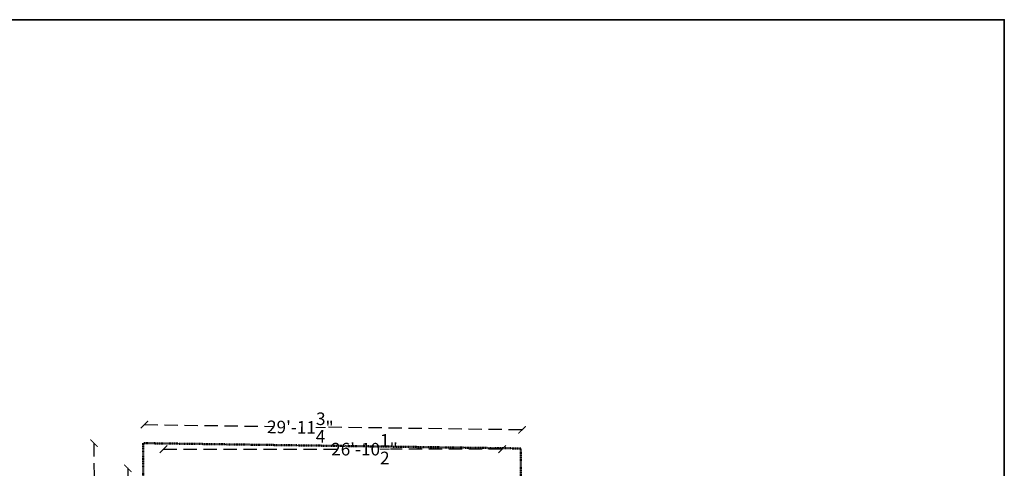
# Model space of a CAD drawing. Units: inches. Extents: x -16911 to -9621, y -48626 to -46270.
# Tile 16 of 20: x -10695 to -9757, y -47771 to -47344. Entities that reach past the tile are written whole.
import ezdxf

# ---------------------------------------------------------------- set-up
doc = ezdxf.new("R2010")
doc.units = ezdxf.units.IN
for name, pattern in [('DASHDOT', [1, 0.5, -0.25, 0, -0.25]), ('DASHED', [19.05, 12.7, -6.35]), ('DOT2', [3.175, 0, -3.175])]:
    doc.linetypes.add(name, pattern=pattern)
for name, color, linetype, lineweight in [('A-ANNO-DIMS', 2, 'Continuous', 13), ('A-WALL', 7, 'Continuous', 35), ('C-PROP', 6, 'DASHDOT', 50)]:
    doc.layers.add(name, color=color, linetype=linetype, lineweight=lineweight)
doc.styles.add('style9', font='swisscl.ttf', dxfattribs={"height": 12})
doc.dimstyles.new('Dim9', dxfattribs={"dimtxt": 10, "dimasz": 0.199219, "dimexe": 1, "dimexo": 0.5, "dimgap": 1, "dimtad": 0, "dimdec": 1, "dimzin": 0, "dimdsep": 46, "dimlunit": 4, "dimtxsty": 'style9', "dimblk": 'ARCHTICK', "dimcen": 0.09, "dimclrd": 256, "dimclrt": 256, "dimadec": 0, "dimazin": 0, "dimtfac": 1, "dimtdec": 1, "dimtix": 1, "dimtofl": 0, "dimtmove": 1, "dimatfit": 3, "dimfxl": 9, "dimtolj": 1, "dimtzin": 0, "dimlwd": -1, "dimarcsym": 0})

# ---------------------------------------------------------------- blocks, each defined once
blk = doc.blocks.new('_ArchTick')
at = {"color": 0, "linetype": 'ByBlock', "const_width": 0.15}
blk.add_lwpolyline([(-0.5, -0.5), (0.5, 0.5)], dxfattribs=at)
blk = doc.blocks.new('*D23')
at = {"layer": 'A-ANNO-DIMS', "color": 0, "linetype": 'DOT2', "lineweight": -2, "transparency": 16777216}
for p, q in [((-10576.06, -47729.98), (-10576.04, -47728.79)), ((-10216.4, -47735.03), (-10216.38, -47733.84))]:
    blk.add_line(p, q, dxfattribs=at)
at = {"layer": 'A-ANNO-DIMS', "color": 0, "linetype": 'DASHED', "lineweight": 25, "transparency": 16777216}
for p, q in [((-10576.06, -47729.79), (-10452.32, -47731.53)), ((-10216.39, -47734.84), (-10402.73, -47732.22))]:
    blk.add_line(p, q, dxfattribs=at)
at = {"layer": 'Defpoints', "color": 0, "transparency": 16777216}
for p in [(-10576.25, -47743.71), (-10216.39, -47734.84), (-10216.59, -47748.75)]:
    blk.add_point(p, dxfattribs=at)
at = {"layer": 'A-ANNO-DIMS', "color": 0, "lineweight": 25, "transparency": 16777216, "xscale": 7, "yscale": 7, "zscale": 7}
for p, rotation in [((-10576.06, -47729.79), 179.1963905603631), ((-10216.39, -47734.84), 359.196390560363)]:
    blk.add_blockref('_ArchTick', p, dxfattribs=dict(at, rotation=rotation))
at = {"layer": 'A-ANNO-DIMS', "color": 0, "transparency": 16777216, "insert": (-10427.53, -47732.32), "char_height": 12, "attachment_point": 5, "rotation": 359.19639, "style": 'style9'}
blk.add_mtext('\\A1;29\'-11{\\H1x;\\S3/4;}"', dxfattribs=at)
blk = doc.blocks.new('*D24')
at = {"layer": 'A-ANNO-DIMS', "color": 0, "linetype": 'DOT2', "lineweight": -2, "transparency": 16777216}
for p, q in [((-10623.85, -47747.46), (-10625.04, -47747.46)), ((-10623.49, -48347.46), (-10624.67, -48347.46))]:
    blk.add_line(p, q, dxfattribs=at)
at = {"layer": 'A-ANNO-DIMS', "color": 0, "linetype": 'DASHED', "lineweight": 25, "transparency": 16777216}
for p, q in [((-10624.04, -47747.46), (-10623.86, -48038.62)), ((-10623.67, -48347.46), (-10623.85, -48056.3))]:
    blk.add_line(p, q, dxfattribs=at)
at = {"layer": 'Defpoints', "color": 0, "transparency": 16777216}
for p in [(-10624.04, -47747.46), (-10605.22, -47747.45), (-10604.86, -48347.45)]:
    blk.add_point(p, dxfattribs=at)
at = {"layer": 'A-ANNO-DIMS', "color": 0, "lineweight": 25, "transparency": 16777216, "xscale": 7, "yscale": 7, "zscale": 7}
for p, rotation in [((-10624.04, -47747.46), 90.0346840750536), ((-10623.67, -48347.46), 270.0346840750536)]:
    blk.add_blockref('_ArchTick', p, dxfattribs=dict(at, rotation=rotation))
at = {"layer": 'A-ANNO-DIMS', "color": 0, "transparency": 16777216, "insert": (-10623.85, -48047.46), "char_height": 12, "attachment_point": 5, "rotation": 270.03468, "style": 'style9'}
blk.add_mtext("\\A1;50'", dxfattribs=at)
blk = doc.blocks.new('*D25')
at = {"layer": 'A-ANNO-DIMS', "color": 0, "linetype": 'DOT2', "lineweight": -2, "transparency": 16777216}
for p, q in [((-10557.82, -47752.97), (-10557.82, -47754.16)), ((-10235.27, -47752.97), (-10235.27, -47754.16))]:
    blk.add_line(p, q, dxfattribs=at)
at = {"layer": 'A-ANNO-DIMS', "color": 0, "linetype": 'DASHED', "lineweight": 25, "transparency": 16777216}
for p, q in [((-10557.82, -47753.16), (-10391.04, -47753.16)), ((-10235.27, -47753.16), (-10341.77, -47753.16))]:
    blk.add_line(p, q, dxfattribs=at)
at = {"layer": 'Defpoints', "color": 0, "transparency": 16777216}
for p in [(-10557.82, -47729.92), (-10235.27, -47729.92), (-10235.27, -47753.16)]:
    blk.add_point(p, dxfattribs=at)
at = {"layer": 'A-ANNO-DIMS', "color": 0, "lineweight": 25, "transparency": 16777216, "xscale": 7, "yscale": 7, "zscale": 7, "rotation": 180}
blk.add_blockref('_ArchTick', (-10557.82, -47753.16), dxfattribs=at)
at = {"layer": 'A-ANNO-DIMS', "color": 0, "lineweight": 25, "transparency": 16777216, "xscale": 7, "yscale": 7, "zscale": 7}
blk.add_blockref('_ArchTick', (-10235.27, -47753.16), dxfattribs=at)
at = {"layer": 'A-ANNO-DIMS', "color": 0, "transparency": 16777216, "insert": (-10366.41, -47753.16), "char_height": 12, "attachment_point": 5, "style": 'style9'}
blk.add_mtext('\\A1;26\'-10{\\H1x;\\S1/2;}"', dxfattribs=at)
blk = doc.blocks.new('*D26')
at = {"layer": 'A-ANNO-DIMS', "color": 0, "linetype": 'DOT2', "lineweight": -2, "transparency": 16777216}
for p, q in [((-10591.56, -47771.49), (-10592.75, -47771.49)), ((-10591.56, -48329.45), (-10592.75, -48329.45))]:
    blk.add_line(p, q, dxfattribs=at)
at = {"layer": 'A-ANNO-DIMS', "color": 0, "linetype": 'DASHED', "lineweight": 25, "transparency": 16777216}
for p, q in [((-10591.75, -47771.49), (-10591.75, -48032.84)), ((-10591.75, -48329.45), (-10591.75, -48068.11))]:
    blk.add_line(p, q, dxfattribs=at)
at = {"layer": 'Defpoints', "color": 0, "transparency": 16777216}
for p in [(-10557.82, -47771.49), (-10591.75, -48329.45), (-10557.82, -48329.45)]:
    blk.add_point(p, dxfattribs=at)
at = {"layer": 'A-ANNO-DIMS', "color": 0, "lineweight": 25, "transparency": 16777216, "xscale": 7, "yscale": 7, "zscale": 7}
for p, rotation in [((-10591.75, -47771.49), 90), ((-10591.75, -48329.45), 270)]:
    blk.add_blockref('_ArchTick', p, dxfattribs=dict(at, rotation=rotation))
at = {"layer": 'A-ANNO-DIMS', "color": 0, "transparency": 16777216, "insert": (-10591.75, -48050.47), "char_height": 12, "attachment_point": 5, "rotation": 90, "style": 'style9'}
blk.add_mtext('\\A1;46\'-6"', dxfattribs=at)

msp = doc.modelspace()

# ---------------------------------------------------------------- linework, layer by layer
at = {"layer": 'A-WALL'}
msp.add_lwpolyline([(-13429.245, -47344.007), (-9756.987, -47344.007), (-9756.987, -48625.922), (-13429.245, -48625.922)], close=True, dxfattribs=at)
at = {"layer": 'C-PROP'}
msp.add_lwpolyline([(-10576.824, -48347.448), (-10216.642, -48353.673), (-10216.081, -48325.085), (-10216.744, -48240.245), (-10217.91, -47994.15), (-10217.524, -47752.494), (-10577.187, -47747.449), (-10576.649, -48147.594)], close=True, dxfattribs=at)

# ---------------------------------------------------------------- dimensions: what is measured, and where the dimension line sits
at = {"layer": 'A-ANNO-DIMS'}
dim = msp.add_linear_dim(base=(-10216.393, -47734.838), p1=(-10576.251, -47743.708), p2=(-10216.588, -47748.753), angle=359.196391, dimstyle='Dim9', override={"dimtxt": 12, "dimasz": 7, "dimdec": 2, "dimclrd": 0, "dimclre": 0, "dimclrt": 0, "dimtdec": 2, "dimfxl": 0.1875, "dimfxlon": 1, "dimlwd": 25, "dimarcsym": 2}, dxfattribs=at)
dim.commit()
dim.dimension.update_dxf_attribs({"geometry": '*D23', "text_midpoint": (-10427.529, -47732.315), "dimtype": 161})
dim = msp.add_linear_dim(base=(-10235.274, -47753.155), p1=(-10557.824, -47729.918), p2=(-10235.274, -47729.918), dimstyle='Dim9', override={"dimtxt": 12, "dimasz": 7, "dimdec": 2, "dimclrd": 0, "dimclre": 0, "dimclrt": 0, "dimtdec": 2, "dimfxl": 0.1875, "dimfxlon": 1, "dimlwd": 25, "dimarcsym": 2}, dxfattribs=at)
dim.commit()
dim.dimension.update_dxf_attribs({"geometry": '*D25', "text_midpoint": (-10366.408, -47753.155), "dimtype": 160})
dim = msp.add_aligned_dim(p1=(-10604.856, -48347.448), p2=(-10605.219, -47747.449), distance=18.817, dimstyle='Dim9', override={"dimtxt": 12, "dimasz": 7, "dimdec": 2, "dimclrd": 0, "dimclre": 0, "dimclrt": 0, "dimtdec": 2, "dimfxl": 0.1875, "dimfxlon": 1, "dimlwd": 25, "dimarcsym": 2}, dxfattribs=at)
dim.commit()
dim.dimension.update_dxf_attribs({"geometry": '*D24', "text_midpoint": (-10623.855, -48047.46)})
dim = msp.add_linear_dim(base=(-10591.752, -48329.448), p1=(-10557.824, -47771.494), p2=(-10557.824, -48329.448), angle=90, dimstyle='Dim9', override={"dimtxt": 12, "dimasz": 7, "dimdec": 2, "dimclrd": 0, "dimclre": 0, "dimclrt": 0, "dimtdec": 2, "dimfxl": 0.1875, "dimfxlon": 1, "dimlwd": 25, "dimarcsym": 2}, dxfattribs=at)
dim.commit()
dim.dimension.update_dxf_attribs({"geometry": '*D26', "text_midpoint": (-10591.752, -48050.471)})

doc.saveas('drawing.dxf')
